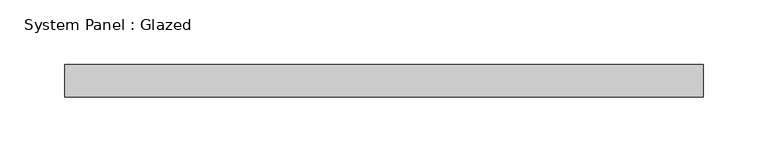
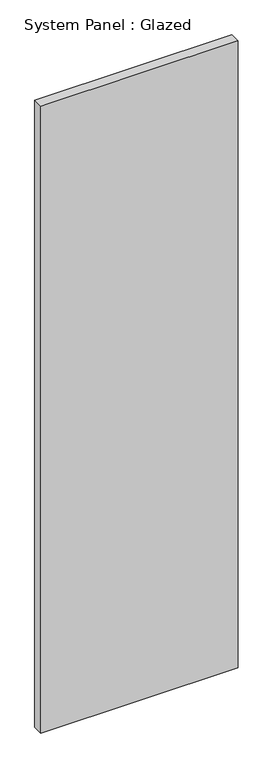
"""IFC4 building model written with IfcOpenShell, lengths in millimetres: plate geometry, System Panel : Glazed."""

from ifc_helpers import new_model, si_unit, origin, origin_with_axes, place, context, project, spatial, polyline, outline, extrude, source, transform, mapped, element, save


def system_panel_glazed_a031bbbc(model_context):
    return source(origin(), model_context, "Body", "SweptSolid", [
        extrude(outline(polyline([(247.65, 19.05), (-247.65, 19.05), (-247.65, 44.45), (247.65, 44.45), (247.65, 19.05)])), origin_with_axes(), (0.0, 0.0, 1.0), 1662.0304763),
    ])


if __name__ == "__main__":
    model = new_model("IFC4")
    model_context = context("Model", 3, world=origin())
    ifc_project = project(units=[si_unit("LENGTHUNIT", "METRE", prefix="MILLI")], contexts=[model_context])
    site = spatial("IfcSite", under=ifc_project)
    building = spatial("IfcBuilding", under=site)
    placement = place(None, origin())
    system_panel_glazed_shape = system_panel_glazed_a031bbbc(model_context)
    element("IfcPlate", 1, ObjectType="System Panel : Glazed", at=placement, inside=building, context=model_context, shape_type="MappedRepresentation", body=[
        mapped(system_panel_glazed_shape, transform((0.0, 0.0, 0.0), x_axis=(1.0, 0.0, 0.0), y_axis=(0.0, 1.0, 0.0), z_axis=(0.0, 0.0, 1.0))),
    ])
    save(model, "model.ifc")

# Revit data of these elements
# Type "System Panel : Glazed"
#   Construction Type Id = "GSP4R"
#   Analytic Construction = "1/8 in Pilkington single glazing"
#   Visual Light Transmittance = 0.9
#   Solar Heat Gain Coefficient = 0.86
#   Heat Transfer Coefficient (U) = 1.18115 BTU/(h·ft²·°F)
#   Define Thermal Properties by = 1
# Element 1 (IfcPlate, "System Panel : Glazed")
#   Materials on its faces: "Glass"
# Materials
#   "Glass": class "Glass", colour RGB 0 128 192, transparency 0.75, Description = "Soda Lime Glass", Cost = 0
